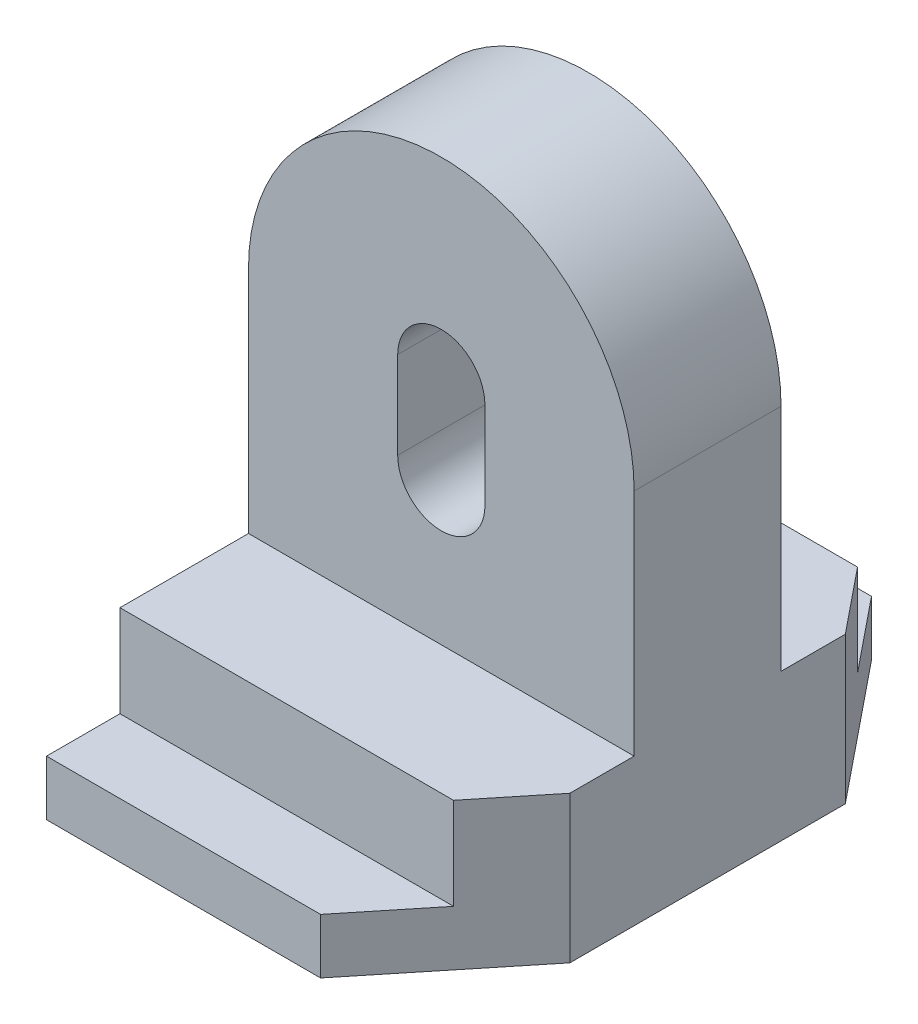
ISO-10303-21;
HEADER;
FILE_DESCRIPTION(('STEP AP214'),'2;1');
FILE_NAME('part.step','',(''),(''),'','','');
FILE_SCHEMA(('AUTOMOTIVE_DESIGN { 1 0 10303 214 1 1 1 1 }'));
ENDSEC;
DATA;
#1=APPLICATION_CONTEXT('core data for automotive mechanical design processes');
#2=APPLICATION_PROTOCOL_DEFINITION('international standard','automotive_design',2000,#1);
#3=PRODUCT_CONTEXT('',#1,'mechanical');
#4=PRODUCT('Part','Part','',(#3));
#5=PRODUCT_RELATED_PRODUCT_CATEGORY('part','',(#4));
#6=PRODUCT_DEFINITION_FORMATION('','',#4);
#7=PRODUCT_DEFINITION_CONTEXT('part definition',#1,'design');
#8=PRODUCT_DEFINITION('design','',#6,#7);
#9=PRODUCT_DEFINITION_SHAPE('','',#8);
#10=(LENGTH_UNIT() NAMED_UNIT(*) SI_UNIT(.MILLI.,.METRE.));
#11=(NAMED_UNIT(*) PLANE_ANGLE_UNIT() SI_UNIT($,.RADIAN.));
#12=(NAMED_UNIT(*) SI_UNIT($,.STERADIAN.) SOLID_ANGLE_UNIT());
#13=UNCERTAINTY_MEASURE_WITH_UNIT(LENGTH_MEASURE(1.E-05),#10,'distance_accuracy_value','');
#14=(GEOMETRIC_REPRESENTATION_CONTEXT(3) GLOBAL_UNCERTAINTY_ASSIGNED_CONTEXT((#13)) GLOBAL_UNIT_ASSIGNED_CONTEXT((#10,
#11,#12)) REPRESENTATION_CONTEXT('',''));
#15=CARTESIAN_POINT('',(0.,0.,0.));
#16=DIRECTION('',(0.,0.,1.));
#17=DIRECTION('',(1.,0.,0.));
#18=AXIS2_PLACEMENT_3D('',#15,#16,#17);
#19=CARTESIAN_POINT('',(42.,32.,-16.));
#20=DIRECTION('',(0.,0.,1.));
#21=DIRECTION('',(1.,0.,0.));
#22=AXIS2_PLACEMENT_3D('',#19,#20,#21);
#23=PLANE('',#22);
#24=DIRECTION('',(0.,-1.,0.));
#25=VECTOR('',#24,1.);
#26=CARTESIAN_POINT('',(9.49999999999999,82.,-16.));
#27=LINE('',#26,#25);
#28=CARTESIAN_POINT('',(9.49999999999999,82.,-16.));
#29=VERTEX_POINT('',#28);
#30=CARTESIAN_POINT('',(9.5,63.,-16.));
#31=VERTEX_POINT('',#30);
#32=EDGE_CURVE('E344',#29,#31,#27,.T.);
#33=ORIENTED_EDGE('',*,*,#32,.F.);
#34=CARTESIAN_POINT('',(0.,82.,-16.));
#35=DIRECTION('',(0.,0.,-1.));
#36=DIRECTION('',(-1.,0.,0.));
#37=AXIS2_PLACEMENT_3D('',#34,#35,#36);
#38=CIRCLE('',#37,9.5);
#39=CARTESIAN_POINT('',(-9.50000000000001,82.,-16.));
#40=VERTEX_POINT('',#39);
#41=EDGE_CURVE('E345',#40,#29,#38,.T.);
#42=ORIENTED_EDGE('',*,*,#41,.F.);
#43=DIRECTION('',(0.,1.,0.));
#44=VECTOR('',#43,1.);
#45=CARTESIAN_POINT('',(-9.50000000000001,82.,-16.));
#46=LINE('',#45,#44);
#47=CARTESIAN_POINT('',(-9.5,63.,-16.));
#48=VERTEX_POINT('',#47);
#49=EDGE_CURVE('E292',#48,#40,#46,.T.);
#50=ORIENTED_EDGE('',*,*,#49,.F.);
#51=CARTESIAN_POINT('',(0.,63.,-16.));
#52=DIRECTION('',(0.,0.,-1.));
#53=DIRECTION('',(-1.,0.,0.));
#54=AXIS2_PLACEMENT_3D('',#51,#52,#53);
#55=CIRCLE('',#54,9.5);
#56=EDGE_CURVE('E347',#31,#48,#55,.T.);
#57=ORIENTED_EDGE('',*,*,#56,.F.);
#58=EDGE_LOOP('',(#33,#42,#50,#57));
#59=FACE_BOUND('',#58,.T.);
#60=DIRECTION('',(0.,1.,0.));
#61=VECTOR('',#60,1.);
#62=CARTESIAN_POINT('',(-42.,32.,-16.));
#63=LINE('',#62,#61);
#64=CARTESIAN_POINT('',(-42.,32.,-16.));
#65=VERTEX_POINT('',#64);
#66=CARTESIAN_POINT('',(-42.,82.,-16.));
#67=VERTEX_POINT('',#66);
#68=EDGE_CURVE('E225',#65,#67,#63,.T.);
#69=ORIENTED_EDGE('',*,*,#68,.T.);
#70=CARTESIAN_POINT('',(0.,82.,-16.));
#71=DIRECTION('',(0.,0.,-1.));
#72=DIRECTION('',(-1.,0.,0.));
#73=AXIS2_PLACEMENT_3D('',#70,#71,#72);
#74=CIRCLE('',#73,42.);
#75=CARTESIAN_POINT('',(42.,82.,-16.));
#76=VERTEX_POINT('',#75);
#77=EDGE_CURVE('E291',#67,#76,#74,.T.);
#78=ORIENTED_EDGE('',*,*,#77,.T.);
#79=DIRECTION('',(0.,1.,0.));
#80=VECTOR('',#79,1.);
#81=CARTESIAN_POINT('',(42.,32.,-16.));
#82=LINE('',#81,#80);
#83=CARTESIAN_POINT('',(42.,32.,-16.));
#84=VERTEX_POINT('',#83);
#85=EDGE_CURVE('E206',#84,#76,#82,.T.);
#86=ORIENTED_EDGE('',*,*,#85,.F.);
#87=DIRECTION('',(-1.,0.,0.));
#88=VECTOR('',#87,1.);
#89=CARTESIAN_POINT('',(42.,32.,-16.));
#90=LINE('',#89,#88);
#91=EDGE_CURVE('E252',#84,#65,#90,.T.);
#92=ORIENTED_EDGE('',*,*,#91,.T.);
#93=EDGE_LOOP('',(#69,#78,#86,#92));
#94=FACE_BOUND('',#93,.T.);
#95=ADVANCED_FACE('F60',(#59,#94),#23,.F.);
#96=CARTESIAN_POINT('',(42.,32.,16.));
#97=DIRECTION('',(0.,0.,-1.));
#98=DIRECTION('',(-1.,0.,0.));
#99=AXIS2_PLACEMENT_3D('',#96,#97,#98);
#100=PLANE('',#99);
#101=DIRECTION('',(0.,1.,0.));
#102=VECTOR('',#101,1.);
#103=CARTESIAN_POINT('',(-9.49999999999998,32.,16.));
#104=LINE('',#103,#102);
#105=CARTESIAN_POINT('',(-9.5,63.,16.));
#106=VERTEX_POINT('',#105);
#107=CARTESIAN_POINT('',(-9.50000000000001,82.,16.));
#108=VERTEX_POINT('',#107);
#109=EDGE_CURVE('E275',#106,#108,#104,.T.);
#110=ORIENTED_EDGE('',*,*,#109,.T.);
#111=CARTESIAN_POINT('',(0.,82.,16.));
#112=DIRECTION('',(0.,0.,-1.));
#113=DIRECTION('',(-1.,0.,0.));
#114=AXIS2_PLACEMENT_3D('',#111,#112,#113);
#115=CIRCLE('',#114,9.5);
#116=CARTESIAN_POINT('',(9.49999999999999,82.,16.));
#117=VERTEX_POINT('',#116);
#118=EDGE_CURVE('E186',#108,#117,#115,.T.);
#119=ORIENTED_EDGE('',*,*,#118,.T.);
#120=DIRECTION('',(0.,-1.,0.));
#121=VECTOR('',#120,1.);
#122=CARTESIAN_POINT('',(9.50000000000001,32.,16.));
#123=LINE('',#122,#121);
#124=CARTESIAN_POINT('',(9.5,63.,16.));
#125=VERTEX_POINT('',#124);
#126=EDGE_CURVE('E266',#117,#125,#123,.T.);
#127=ORIENTED_EDGE('',*,*,#126,.T.);
#128=CARTESIAN_POINT('',(0.,63.,16.));
#129=DIRECTION('',(0.,0.,-1.));
#130=DIRECTION('',(-1.,0.,0.));
#131=AXIS2_PLACEMENT_3D('',#128,#129,#130);
#132=CIRCLE('',#131,9.5);
#133=EDGE_CURVE('E267',#125,#106,#132,.T.);
#134=ORIENTED_EDGE('',*,*,#133,.T.);
#135=EDGE_LOOP('',(#110,#119,#127,#134));
#136=FACE_BOUND('',#135,.T.);
#137=CARTESIAN_POINT('',(0.,82.,16.));
#138=DIRECTION('',(0.,0.,-1.));
#139=DIRECTION('',(-1.,0.,0.));
#140=AXIS2_PLACEMENT_3D('',#137,#138,#139);
#141=CIRCLE('',#140,42.);
#142=CARTESIAN_POINT('',(-42.,82.,16.));
#143=VERTEX_POINT('',#142);
#144=CARTESIAN_POINT('',(42.,82.,16.));
#145=VERTEX_POINT('',#144);
#146=EDGE_CURVE('E212',#143,#145,#141,.T.);
#147=ORIENTED_EDGE('',*,*,#146,.F.);
#148=DIRECTION('',(0.,-1.,0.));
#149=VECTOR('',#148,1.);
#150=CARTESIAN_POINT('',(-42.,32.,16.));
#151=LINE('',#150,#149);
#152=CARTESIAN_POINT('',(-42.,32.,16.));
#153=VERTEX_POINT('',#152);
#154=EDGE_CURVE('E223',#143,#153,#151,.T.);
#155=ORIENTED_EDGE('',*,*,#154,.T.);
#156=DIRECTION('',(-1.,0.,0.));
#157=VECTOR('',#156,1.);
#158=CARTESIAN_POINT('',(42.,32.,16.));
#159=LINE('',#158,#157);
#160=CARTESIAN_POINT('',(42.,32.,16.));
#161=VERTEX_POINT('',#160);
#162=EDGE_CURVE('E247',#161,#153,#159,.T.);
#163=ORIENTED_EDGE('',*,*,#162,.F.);
#164=DIRECTION('',(0.,-1.,0.));
#165=VECTOR('',#164,1.);
#166=CARTESIAN_POINT('',(42.,32.,16.));
#167=LINE('',#166,#165);
#168=EDGE_CURVE('E199',#145,#161,#167,.T.);
#169=ORIENTED_EDGE('',*,*,#168,.F.);
#170=EDGE_LOOP('',(#147,#155,#163,#169));
#171=FACE_BOUND('',#170,.T.);
#172=ADVANCED_FACE('F280',(#136,#171),#100,.F.);
#173=CARTESIAN_POINT('',(42.,0.,-60.));
#174=DIRECTION('',(0.,0.,1.));
#175=DIRECTION('',(1.,0.,0.));
#176=AXIS2_PLACEMENT_3D('',#173,#174,#175);
#177=PLANE('',#176);
#178=DIRECTION('',(-1.,0.,0.));
#179=VECTOR('',#178,1.);
#180=CARTESIAN_POINT('',(42.,12.,-60.));
#181=LINE('',#180,#179);
#182=CARTESIAN_POINT('',(17.7064790041495,12.,-60.));
#183=VERTEX_POINT('',#182);
#184=CARTESIAN_POINT('',(-42.,12.,-60.));
#185=VERTEX_POINT('',#184);
#186=EDGE_CURVE('E259',#183,#185,#181,.T.);
#187=ORIENTED_EDGE('',*,*,#186,.F.);
#188=DIRECTION('',(0.,1.,0.));
#189=VECTOR('',#188,1.);
#190=CARTESIAN_POINT('',(17.7064790041495,-8.,-60.));
#191=LINE('',#190,#189);
#192=CARTESIAN_POINT('',(17.7064790041495,0.,-60.));
#193=VERTEX_POINT('',#192);
#194=EDGE_CURVE('E393',#193,#183,#191,.T.);
#195=ORIENTED_EDGE('',*,*,#194,.F.);
#196=DIRECTION('',(-1.,0.,0.));
#197=VECTOR('',#196,1.);
#198=CARTESIAN_POINT('',(42.,0.,-60.));
#199=LINE('',#198,#197);
#200=CARTESIAN_POINT('',(-42.,0.,-60.));
#201=VERTEX_POINT('',#200);
#202=EDGE_CURVE('E204',#193,#201,#199,.T.);
#203=ORIENTED_EDGE('',*,*,#202,.T.);
#204=DIRECTION('',(0.,1.,0.));
#205=VECTOR('',#204,1.);
#206=CARTESIAN_POINT('',(-42.,0.,-60.));
#207=LINE('',#206,#205);
#208=EDGE_CURVE('E209',#201,#185,#207,.T.);
#209=ORIENTED_EDGE('',*,*,#208,.T.);
#210=EDGE_LOOP('',(#187,#195,#203,#209));
#211=FACE_BOUND('',#210,.T.);
#212=ADVANCED_FACE('F56',(#211),#177,.F.);
#213=CARTESIAN_POINT('',(42.,12.,-60.));
#214=DIRECTION('',(0.,-1.,0.));
#215=DIRECTION('',(0.,0.,-1.));
#216=AXIS2_PLACEMENT_3D('',#213,#214,#215);
#217=PLANE('',#216);
#218=DIRECTION('',(-1.,0.,0.));
#219=VECTOR('',#218,1.);
#220=CARTESIAN_POINT('',(42.,12.,-44.));
#221=LINE('',#220,#219);
#222=CARTESIAN_POINT('',(30.6630235352698,12.,-44.));
#223=VERTEX_POINT('',#222);
#224=CARTESIAN_POINT('',(-42.,12.,-44.));
#225=VERTEX_POINT('',#224);
#226=EDGE_CURVE('E260',#223,#225,#221,.T.);
#227=ORIENTED_EDGE('',*,*,#226,.F.);
#228=DIRECTION('',(-0.629320391049842,0.,-0.777145961456967));
#229=VECTOR('',#228,1.);
#230=CARTESIAN_POINT('',(27.3277859889929,12.,-48.1186753622662));
#231=LINE('',#230,#229);
#232=EDGE_CURVE('E338',#223,#183,#231,.T.);
#233=ORIENTED_EDGE('',*,*,#232,.T.);
#234=ORIENTED_EDGE('',*,*,#186,.T.);
#235=DIRECTION('',(0.,0.,1.));
#236=VECTOR('',#235,1.);
#237=CARTESIAN_POINT('',(-42.,12.,-60.));
#238=LINE('',#237,#236);
#239=EDGE_CURVE('E213',#185,#225,#238,.T.);
#240=ORIENTED_EDGE('',*,*,#239,.T.);
#241=EDGE_LOOP('',(#227,#233,#234,#240));
#242=FACE_BOUND('',#241,.T.);
#243=ADVANCED_FACE('F385',(#242),#217,.F.);
#244=CARTESIAN_POINT('',(42.,12.,-44.));
#245=DIRECTION('',(0.,0.,1.));
#246=DIRECTION('',(1.,0.,0.));
#247=AXIS2_PLACEMENT_3D('',#244,#245,#246);
#248=PLANE('',#247);
#249=DIRECTION('',(-1.,0.,0.));
#250=VECTOR('',#249,1.);
#251=CARTESIAN_POINT('',(42.,32.,-44.));
#252=LINE('',#251,#250);
#253=CARTESIAN_POINT('',(30.6630235352698,32.,-44.));
#254=VERTEX_POINT('',#253);
#255=CARTESIAN_POINT('',(-42.,32.,-44.));
#256=VERTEX_POINT('',#255);
#257=EDGE_CURVE('E254',#254,#256,#252,.T.);
#258=ORIENTED_EDGE('',*,*,#257,.F.);
#259=DIRECTION('',(0.,-1.,0.));
#260=VECTOR('',#259,1.);
#261=CARTESIAN_POINT('',(30.6630235352698,12.,-44.));
#262=LINE('',#261,#260);
#263=EDGE_CURVE('E335',#254,#223,#262,.T.);
#264=ORIENTED_EDGE('',*,*,#263,.T.);
#265=ORIENTED_EDGE('',*,*,#226,.T.);
#266=DIRECTION('',(0.,1.,0.));
#267=VECTOR('',#266,1.);
#268=CARTESIAN_POINT('',(-42.,12.,-44.));
#269=LINE('',#268,#267);
#270=EDGE_CURVE('E220',#225,#256,#269,.T.);
#271=ORIENTED_EDGE('',*,*,#270,.T.);
#272=EDGE_LOOP('',(#258,#264,#265,#271));
#273=FACE_BOUND('',#272,.T.);
#274=ADVANCED_FACE('F377',(#273),#248,.F.);
#275=CARTESIAN_POINT('',(42.,32.,-44.));
#276=DIRECTION('',(0.,-1.,0.));
#277=DIRECTION('',(0.,0.,-1.));
#278=AXIS2_PLACEMENT_3D('',#275,#276,#277);
#279=PLANE('',#278);
#280=DIRECTION('',(0.,0.,1.));
#281=VECTOR('',#280,1.);
#282=CARTESIAN_POINT('',(42.,32.,-44.));
#283=LINE('',#282,#281);
#284=CARTESIAN_POINT('',(42.,32.,-30.));
#285=VERTEX_POINT('',#284);
#286=EDGE_CURVE('E241',#285,#84,#283,.T.);
#287=ORIENTED_EDGE('',*,*,#286,.F.);
#288=DIRECTION('',(0.629320391049842,0.,0.777145961456967));
#289=VECTOR('',#288,1.);
#290=CARTESIAN_POINT('',(42.,32.,-30.));
#291=LINE('',#290,#289);
#292=EDGE_CURVE('E72',#254,#285,#291,.T.);
#293=ORIENTED_EDGE('',*,*,#292,.F.);
#294=ORIENTED_EDGE('',*,*,#257,.T.);
#295=DIRECTION('',(0.,0.,1.));
#296=VECTOR('',#295,1.);
#297=CARTESIAN_POINT('',(-42.,32.,-44.));
#298=LINE('',#297,#296);
#299=EDGE_CURVE('E219',#256,#65,#298,.T.);
#300=ORIENTED_EDGE('',*,*,#299,.T.);
#301=ORIENTED_EDGE('',*,*,#91,.F.);
#302=EDGE_LOOP('',(#287,#293,#294,#300,#301));
#303=FACE_BOUND('',#302,.T.);
#304=ADVANCED_FACE('F376',(#303),#279,.F.);
#305=CARTESIAN_POINT('',(42.,32.,44.));
#306=DIRECTION('',(0.,-1.,0.));
#307=DIRECTION('',(0.,0.,-1.));
#308=AXIS2_PLACEMENT_3D('',#305,#306,#307);
#309=PLANE('',#308);
#310=DIRECTION('',(-1.,0.,0.));
#311=VECTOR('',#310,1.);
#312=CARTESIAN_POINT('',(42.,32.,44.));
#313=LINE('',#312,#311);
#314=CARTESIAN_POINT('',(30.6630235352698,32.,44.));
#315=VERTEX_POINT('',#314);
#316=CARTESIAN_POINT('',(-42.,32.,44.));
#317=VERTEX_POINT('',#316);
#318=EDGE_CURVE('E194',#315,#317,#313,.T.);
#319=ORIENTED_EDGE('',*,*,#318,.F.);
#320=DIRECTION('',(-0.629320391049841,0.,0.777145961456968));
#321=VECTOR('',#320,1.);
#322=CARTESIAN_POINT('',(42.,32.,30.));
#323=LINE('',#322,#321);
#324=CARTESIAN_POINT('',(42.,32.,30.));
#325=VERTEX_POINT('',#324);
#326=EDGE_CURVE('E177',#325,#315,#323,.T.);
#327=ORIENTED_EDGE('',*,*,#326,.F.);
#328=DIRECTION('',(0.,0.,1.));
#329=VECTOR('',#328,1.);
#330=CARTESIAN_POINT('',(42.,32.,44.));
#331=LINE('',#330,#329);
#332=EDGE_CURVE('E195',#161,#325,#331,.T.);
#333=ORIENTED_EDGE('',*,*,#332,.F.);
#334=ORIENTED_EDGE('',*,*,#162,.T.);
#335=DIRECTION('',(0.,0.,1.));
#336=VECTOR('',#335,1.);
#337=CARTESIAN_POINT('',(-42.,32.,44.));
#338=LINE('',#337,#336);
#339=EDGE_CURVE('E230',#153,#317,#338,.T.);
#340=ORIENTED_EDGE('',*,*,#339,.T.);
#341=EDGE_LOOP('',(#319,#327,#333,#334,#340));
#342=FACE_BOUND('',#341,.T.);
#343=ADVANCED_FACE('F189',(#342),#309,.F.);
#344=CARTESIAN_POINT('',(42.,12.,44.));
#345=DIRECTION('',(0.,0.,-1.));
#346=DIRECTION('',(-1.,0.,0.));
#347=AXIS2_PLACEMENT_3D('',#344,#345,#346);
#348=PLANE('',#347);
#349=DIRECTION('',(-1.,0.,0.));
#350=VECTOR('',#349,1.);
#351=CARTESIAN_POINT('',(42.,12.,44.));
#352=LINE('',#351,#350);
#353=CARTESIAN_POINT('',(30.6630235352698,12.,44.));
#354=VERTEX_POINT('',#353);
#355=CARTESIAN_POINT('',(-42.,12.,44.));
#356=VERTEX_POINT('',#355);
#357=EDGE_CURVE('E250',#354,#356,#352,.T.);
#358=ORIENTED_EDGE('',*,*,#357,.F.);
#359=DIRECTION('',(0.,1.,0.));
#360=VECTOR('',#359,1.);
#361=CARTESIAN_POINT('',(30.6630235352698,12.,44.));
#362=LINE('',#361,#360);
#363=EDGE_CURVE('E326',#354,#315,#362,.T.);
#364=ORIENTED_EDGE('',*,*,#363,.T.);
#365=ORIENTED_EDGE('',*,*,#318,.T.);
#366=DIRECTION('',(0.,-1.,0.));
#367=VECTOR('',#366,1.);
#368=CARTESIAN_POINT('',(-42.,12.,44.));
#369=LINE('',#368,#367);
#370=EDGE_CURVE('E228',#317,#356,#369,.T.);
#371=ORIENTED_EDGE('',*,*,#370,.T.);
#372=EDGE_LOOP('',(#358,#364,#365,#371));
#373=FACE_BOUND('',#372,.T.);
#374=ADVANCED_FACE('F324',(#373),#348,.F.);
#375=CARTESIAN_POINT('',(42.,12.,60.));
#376=DIRECTION('',(0.,-1.,0.));
#377=DIRECTION('',(0.,0.,-1.));
#378=AXIS2_PLACEMENT_3D('',#375,#376,#377);
#379=PLANE('',#378);
#380=DIRECTION('',(-1.,0.,0.));
#381=VECTOR('',#380,1.);
#382=CARTESIAN_POINT('',(42.,12.,60.));
#383=LINE('',#382,#381);
#384=CARTESIAN_POINT('',(17.7064790041495,12.,60.));
#385=VERTEX_POINT('',#384);
#386=CARTESIAN_POINT('',(-42.,12.,60.));
#387=VERTEX_POINT('',#386);
#388=EDGE_CURVE('E244',#385,#387,#383,.T.);
#389=ORIENTED_EDGE('',*,*,#388,.F.);
#390=DIRECTION('',(0.629320391049841,0.,-0.777145961456968));
#391=VECTOR('',#390,1.);
#392=CARTESIAN_POINT('',(27.3277859889929,12.,48.1186753622662));
#393=LINE('',#392,#391);
#394=EDGE_CURVE('E328',#385,#354,#393,.T.);
#395=ORIENTED_EDGE('',*,*,#394,.T.);
#396=ORIENTED_EDGE('',*,*,#357,.T.);
#397=DIRECTION('',(0.,0.,1.));
#398=VECTOR('',#397,1.);
#399=CARTESIAN_POINT('',(-42.,12.,60.));
#400=LINE('',#399,#398);
#401=EDGE_CURVE('E235',#356,#387,#400,.T.);
#402=ORIENTED_EDGE('',*,*,#401,.T.);
#403=EDGE_LOOP('',(#389,#395,#396,#402));
#404=FACE_BOUND('',#403,.T.);
#405=ADVANCED_FACE('F409',(#404),#379,.F.);
#406=CARTESIAN_POINT('',(42.,0.,60.));
#407=DIRECTION('',(0.,0.,-1.));
#408=DIRECTION('',(-1.,0.,0.));
#409=AXIS2_PLACEMENT_3D('',#406,#407,#408);
#410=PLANE('',#409);
#411=DIRECTION('',(-1.,0.,0.));
#412=VECTOR('',#411,1.);
#413=CARTESIAN_POINT('',(42.,0.,60.));
#414=LINE('',#413,#412);
#415=CARTESIAN_POINT('',(17.7064790041495,0.,60.));
#416=VERTEX_POINT('',#415);
#417=CARTESIAN_POINT('',(-42.,0.,60.));
#418=VERTEX_POINT('',#417);
#419=EDGE_CURVE('E242',#416,#418,#414,.T.);
#420=ORIENTED_EDGE('',*,*,#419,.F.);
#421=DIRECTION('',(0.,1.,0.));
#422=VECTOR('',#421,1.);
#423=CARTESIAN_POINT('',(17.7064790041495,-8.00000000000003,60.));
#424=LINE('',#423,#422);
#425=EDGE_CURVE('E192',#416,#385,#424,.T.);
#426=ORIENTED_EDGE('',*,*,#425,.T.);
#427=ORIENTED_EDGE('',*,*,#388,.T.);
#428=DIRECTION('',(0.,-1.,0.));
#429=VECTOR('',#428,1.);
#430=CARTESIAN_POINT('',(-42.,0.,60.));
#431=LINE('',#430,#429);
#432=EDGE_CURVE('E232',#387,#418,#431,.T.);
#433=ORIENTED_EDGE('',*,*,#432,.T.);
#434=EDGE_LOOP('',(#420,#426,#427,#433));
#435=FACE_BOUND('',#434,.T.);
#436=ADVANCED_FACE('F404',(#435),#410,.F.);
#437=CARTESIAN_POINT('',(42.,0.,60.));
#438=DIRECTION('',(0.,1.,0.));
#439=DIRECTION('',(0.,0.,1.));
#440=AXIS2_PLACEMENT_3D('',#437,#438,#439);
#441=PLANE('',#440);
#442=ORIENTED_EDGE('',*,*,#202,.F.);
#443=DIRECTION('',(0.629320391049842,0.,0.777145961456967));
#444=VECTOR('',#443,1.);
#445=CARTESIAN_POINT('',(86.0166420330214,0.,24.3560260867986));
#446=LINE('',#445,#444);
#447=CARTESIAN_POINT('',(42.,0.,-30.));
#448=VERTEX_POINT('',#447);
#449=EDGE_CURVE('E327',#193,#448,#446,.T.);
#450=ORIENTED_EDGE('',*,*,#449,.T.);
#451=DIRECTION('',(0.,0.,-1.));
#452=VECTOR('',#451,1.);
#453=CARTESIAN_POINT('',(42.,0.,60.));
#454=LINE('',#453,#452);
#455=CARTESIAN_POINT('',(42.,0.,30.));
#456=VERTEX_POINT('',#455);
#457=EDGE_CURVE('E205',#456,#448,#454,.T.);
#458=ORIENTED_EDGE('',*,*,#457,.F.);
#459=DIRECTION('',(-0.629320391049841,0.,0.777145961456968));
#460=VECTOR('',#459,1.);
#461=CARTESIAN_POINT('',(27.3277859889929,0.,48.1186753622662));
#462=LINE('',#461,#460);
#463=EDGE_CURVE('E78',#456,#416,#462,.T.);
#464=ORIENTED_EDGE('',*,*,#463,.T.);
#465=ORIENTED_EDGE('',*,*,#419,.T.);
#466=DIRECTION('',(0.,0.,-1.));
#467=VECTOR('',#466,1.);
#468=CARTESIAN_POINT('',(-42.,0.,60.));
#469=LINE('',#468,#467);
#470=EDGE_CURVE('E236',#418,#201,#469,.T.);
#471=ORIENTED_EDGE('',*,*,#470,.T.);
#472=EDGE_LOOP('',(#442,#450,#458,#464,#465,#471));
#473=FACE_BOUND('',#472,.T.);
#474=ADVANCED_FACE('F405',(#473),#441,.F.);
#475=CARTESIAN_POINT('',(42.,0.,0.));
#476=DIRECTION('',(1.,0.,0.));
#477=DIRECTION('',(0.,0.,-1.));
#478=AXIS2_PLACEMENT_3D('',#475,#476,#477);
#479=PLANE('',#478);
#480=DIRECTION('',(0.,-1.,0.));
#481=VECTOR('',#480,1.);
#482=CARTESIAN_POINT('',(42.,0.,-30.));
#483=LINE('',#482,#481);
#484=EDGE_CURVE('E12',#285,#448,#483,.T.);
#485=ORIENTED_EDGE('',*,*,#484,.F.);
#486=ORIENTED_EDGE('',*,*,#286,.T.);
#487=ORIENTED_EDGE('',*,*,#85,.T.);
#488=DIRECTION('',(0.,0.,-1.));
#489=VECTOR('',#488,1.);
#490=CARTESIAN_POINT('',(42.,82.,24.));
#491=LINE('',#490,#489);
#492=EDGE_CURVE('E261',#145,#76,#491,.T.);
#493=ORIENTED_EDGE('',*,*,#492,.F.);
#494=ORIENTED_EDGE('',*,*,#168,.T.);
#495=ORIENTED_EDGE('',*,*,#332,.T.);
#496=DIRECTION('',(0.,1.,0.));
#497=VECTOR('',#496,1.);
#498=CARTESIAN_POINT('',(42.,0.,30.));
#499=LINE('',#498,#497);
#500=EDGE_CURVE('E64',#456,#325,#499,.T.);
#501=ORIENTED_EDGE('',*,*,#500,.F.);
#502=ORIENTED_EDGE('',*,*,#457,.T.);
#503=EDGE_LOOP('',(#485,#486,#487,#493,#494,#495,#501,#502));
#504=FACE_BOUND('',#503,.T.);
#505=ADVANCED_FACE('F197',(#504),#479,.T.);
#506=CARTESIAN_POINT('',(-42.,0.,0.));
#507=DIRECTION('',(1.,0.,0.));
#508=DIRECTION('',(0.,0.,-1.));
#509=AXIS2_PLACEMENT_3D('',#506,#507,#508);
#510=PLANE('',#509);
#511=ORIENTED_EDGE('',*,*,#154,.F.);
#512=DIRECTION('',(0.,0.,-1.));
#513=VECTOR('',#512,1.);
#514=CARTESIAN_POINT('',(-42.,82.,24.));
#515=LINE('',#514,#513);
#516=EDGE_CURVE('E263',#143,#67,#515,.T.);
#517=ORIENTED_EDGE('',*,*,#516,.T.);
#518=ORIENTED_EDGE('',*,*,#68,.F.);
#519=ORIENTED_EDGE('',*,*,#299,.F.);
#520=ORIENTED_EDGE('',*,*,#270,.F.);
#521=ORIENTED_EDGE('',*,*,#239,.F.);
#522=ORIENTED_EDGE('',*,*,#208,.F.);
#523=ORIENTED_EDGE('',*,*,#470,.F.);
#524=ORIENTED_EDGE('',*,*,#432,.F.);
#525=ORIENTED_EDGE('',*,*,#401,.F.);
#526=ORIENTED_EDGE('',*,*,#370,.F.);
#527=ORIENTED_EDGE('',*,*,#339,.F.);
#528=EDGE_LOOP('',(#511,#517,#518,#519,#520,#521,#522,#523,#524,#525,#526,#527));
#529=FACE_BOUND('',#528,.T.);
#530=ADVANCED_FACE('F320',(#529),#510,.F.);
#531=CARTESIAN_POINT('',(0.,82.,24.));
#532=DIRECTION('',(0.,0.,-1.));
#533=DIRECTION('',(-1.,0.,0.));
#534=AXIS2_PLACEMENT_3D('',#531,#532,#533);
#535=CYLINDRICAL_SURFACE('',#534,42.);
#536=ORIENTED_EDGE('',*,*,#146,.T.);
#537=ORIENTED_EDGE('',*,*,#492,.T.);
#538=ORIENTED_EDGE('',*,*,#77,.F.);
#539=ORIENTED_EDGE('',*,*,#516,.F.);
#540=EDGE_LOOP('',(#536,#537,#538,#539));
#541=FACE_BOUND('',#540,.T.);
#542=ADVANCED_FACE('F314',(#541),#535,.T.);
#543=CARTESIAN_POINT('',(0.,82.,24.));
#544=DIRECTION('',(0.,0.,-1.));
#545=DIRECTION('',(-1.,0.,0.));
#546=AXIS2_PLACEMENT_3D('',#543,#544,#545);
#547=CYLINDRICAL_SURFACE('',#546,9.5);
#548=DIRECTION('',(0.,0.,-1.));
#549=VECTOR('',#548,1.);
#550=CARTESIAN_POINT('',(-9.50000000000001,82.,24.));
#551=LINE('',#550,#549);
#552=EDGE_CURVE('E282',#108,#40,#551,.T.);
#553=ORIENTED_EDGE('',*,*,#552,.T.);
#554=ORIENTED_EDGE('',*,*,#41,.T.);
#555=DIRECTION('',(0.,0.,-1.));
#556=VECTOR('',#555,1.);
#557=CARTESIAN_POINT('',(9.49999999999999,82.,24.));
#558=LINE('',#557,#556);
#559=EDGE_CURVE('E288',#117,#29,#558,.T.);
#560=ORIENTED_EDGE('',*,*,#559,.F.);
#561=ORIENTED_EDGE('',*,*,#118,.F.);
#562=EDGE_LOOP('',(#553,#554,#560,#561));
#563=FACE_BOUND('',#562,.T.);
#564=ADVANCED_FACE('F285',(#563),#547,.F.);
#565=CARTESIAN_POINT('',(-9.50000000000001,82.,24.));
#566=DIRECTION('',(-1.,0.,0.));
#567=DIRECTION('',(0.,-1.,0.));
#568=AXIS2_PLACEMENT_3D('',#565,#566,#567);
#569=PLANE('',#568);
#570=DIRECTION('',(0.,0.,-1.));
#571=VECTOR('',#570,1.);
#572=CARTESIAN_POINT('',(-9.5,63.,24.));
#573=LINE('',#572,#571);
#574=EDGE_CURVE('E294',#106,#48,#573,.T.);
#575=ORIENTED_EDGE('',*,*,#574,.T.);
#576=ORIENTED_EDGE('',*,*,#49,.T.);
#577=ORIENTED_EDGE('',*,*,#552,.F.);
#578=ORIENTED_EDGE('',*,*,#109,.F.);
#579=EDGE_LOOP('',(#575,#576,#577,#578));
#580=FACE_BOUND('',#579,.T.);
#581=ADVANCED_FACE('F286',(#580),#569,.F.);
#582=CARTESIAN_POINT('',(0.,63.,24.));
#583=DIRECTION('',(0.,0.,-1.));
#584=DIRECTION('',(-1.,0.,0.));
#585=AXIS2_PLACEMENT_3D('',#582,#583,#584);
#586=CYLINDRICAL_SURFACE('',#585,9.5);
#587=DIRECTION('',(0.,0.,-1.));
#588=VECTOR('',#587,1.);
#589=CARTESIAN_POINT('',(9.5,63.,24.));
#590=LINE('',#589,#588);
#591=EDGE_CURVE('E297',#125,#31,#590,.T.);
#592=ORIENTED_EDGE('',*,*,#591,.T.);
#593=ORIENTED_EDGE('',*,*,#56,.T.);
#594=ORIENTED_EDGE('',*,*,#574,.F.);
#595=ORIENTED_EDGE('',*,*,#133,.F.);
#596=EDGE_LOOP('',(#592,#593,#594,#595));
#597=FACE_BOUND('',#596,.T.);
#598=ADVANCED_FACE('F348',(#597),#586,.F.);
#599=CARTESIAN_POINT('',(9.49999999999999,82.,24.));
#600=DIRECTION('',(1.,0.,0.));
#601=DIRECTION('',(0.,1.,0.));
#602=AXIS2_PLACEMENT_3D('',#599,#600,#601);
#603=PLANE('',#602);
#604=ORIENTED_EDGE('',*,*,#559,.T.);
#605=ORIENTED_EDGE('',*,*,#32,.T.);
#606=ORIENTED_EDGE('',*,*,#591,.F.);
#607=ORIENTED_EDGE('',*,*,#126,.F.);
#608=EDGE_LOOP('',(#604,#605,#606,#607));
#609=FACE_BOUND('',#608,.T.);
#610=ADVANCED_FACE('F354',(#609),#603,.F.);
#611=CARTESIAN_POINT('',(42.,-8.00000000000002,30.));
#612=DIRECTION('',(-0.777145961456968,0.,-0.629320391049841));
#613=DIRECTION('',(-0.629320391049841,0.,0.777145961456968));
#614=AXIS2_PLACEMENT_3D('',#611,#612,#613);
#615=PLANE('',#614);
#616=ORIENTED_EDGE('',*,*,#394,.F.);
#617=ORIENTED_EDGE('',*,*,#425,.F.);
#618=ORIENTED_EDGE('',*,*,#463,.F.);
#619=ORIENTED_EDGE('',*,*,#500,.T.);
#620=ORIENTED_EDGE('',*,*,#326,.T.);
#621=ORIENTED_EDGE('',*,*,#363,.F.);
#622=EDGE_LOOP('',(#616,#617,#618,#619,#620,#621));
#623=FACE_BOUND('',#622,.T.);
#624=ADVANCED_FACE('F179',(#623),#615,.F.);
#625=CARTESIAN_POINT('',(42.,-8.00000000000001,-30.));
#626=DIRECTION('',(-0.777145961456967,0.,0.629320391049842));
#627=DIRECTION('',(0.629320391049842,0.,0.777145961456967));
#628=AXIS2_PLACEMENT_3D('',#625,#626,#627);
#629=PLANE('',#628);
#630=ORIENTED_EDGE('',*,*,#263,.F.);
#631=ORIENTED_EDGE('',*,*,#292,.T.);
#632=ORIENTED_EDGE('',*,*,#484,.T.);
#633=ORIENTED_EDGE('',*,*,#449,.F.);
#634=ORIENTED_EDGE('',*,*,#194,.T.);
#635=ORIENTED_EDGE('',*,*,#232,.F.);
#636=EDGE_LOOP('',(#630,#631,#632,#633,#634,#635));
#637=FACE_BOUND('',#636,.T.);
#638=ADVANCED_FACE('F361',(#637),#629,.F.);
#639=CLOSED_SHELL('',(#95,#172,#212,#243,#274,#304,#343,#374,#405,#436,#474,#505,#530,#542,#564,
#581,#598,#610,#624,#638));
#640=MANIFOLD_SOLID_BREP('B2',#639);
#641=ADVANCED_BREP_SHAPE_REPRESENTATION('',(#18,#640),#14);
#642=SHAPE_DEFINITION_REPRESENTATION(#9,#641);
ENDSEC;
END-ISO-10303-21;
